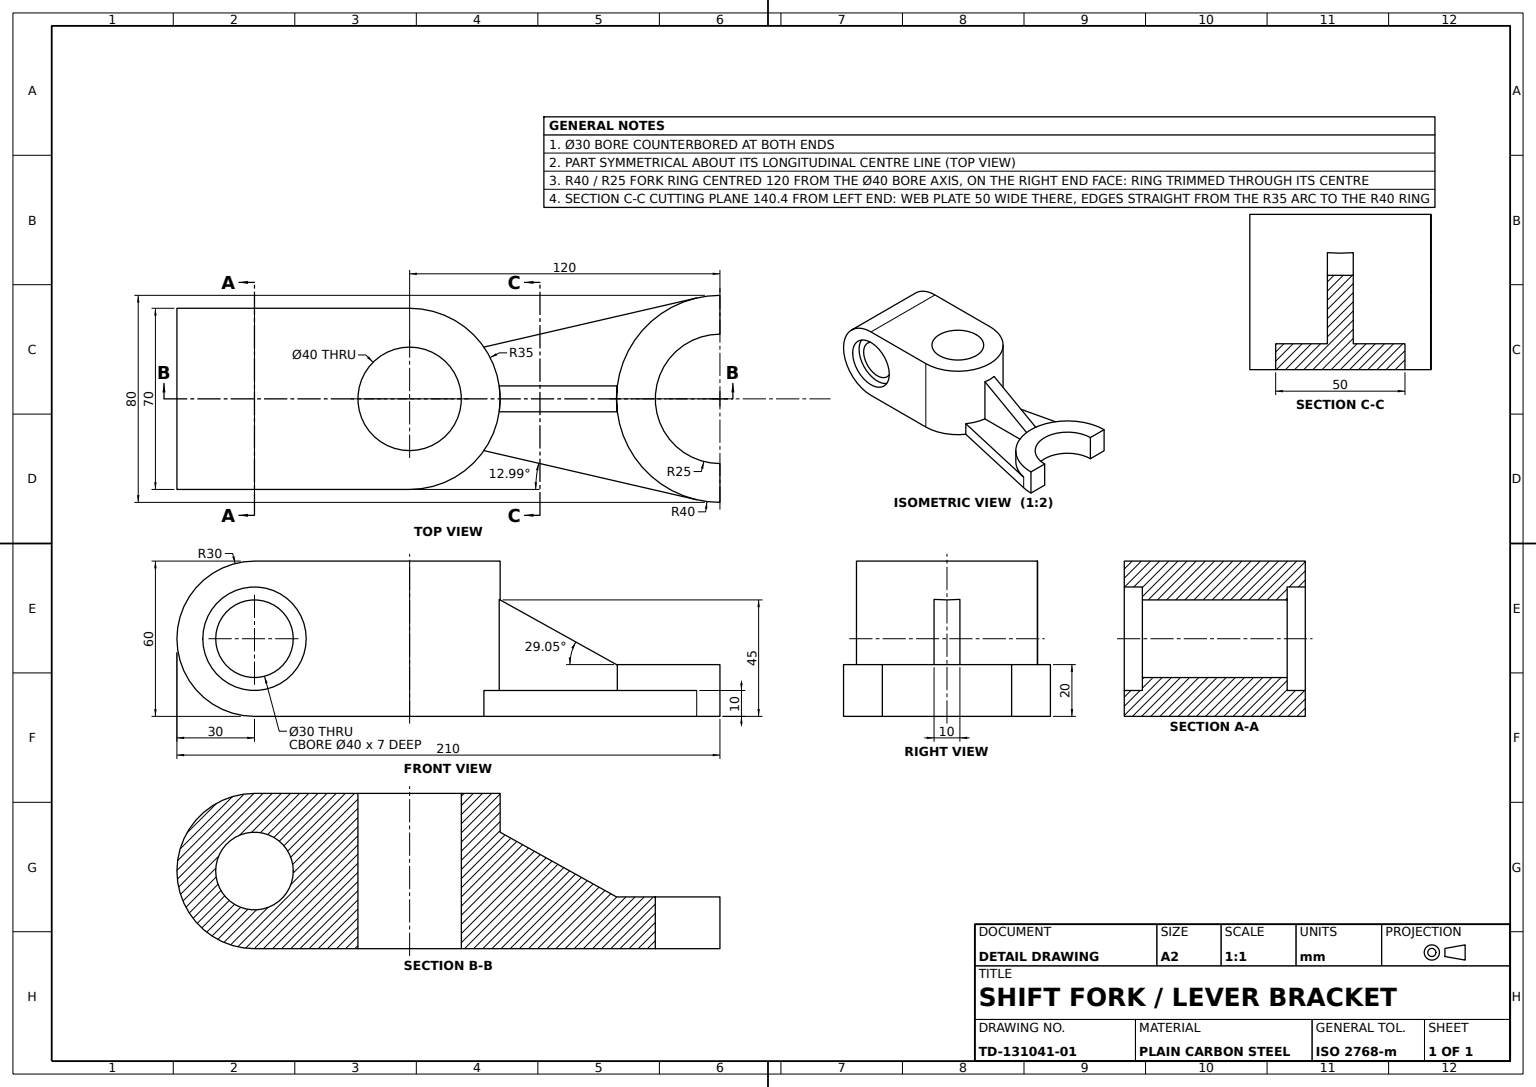
SolidWorks part; units mm, degrees
material "Plain Carbon Steel"
ref_plane "Front Plane" through (0, 0, 0) normal (0, 0, 1) x (1, 0, 0)
ref_plane "Top Plane" through (0, 0, 0) normal (0, 1, 0) x (1, 0, 0)
ref_plane "Right Plane" through (0, 0, 0) normal (1, 0, 0) x (0, 0, -1)
sketch "Base Block Sketch" plane through (0, 0, 0) normal (0, 1, 0) x (1, 0, 0)
  line L0 (0, 35) -> (-90, 35)
  line L1 (-90, 35) -> (-90, -35)
  line L2 (-90, -35) -> (0, -35)
  arc A0 (0, -35) -> (0, 35) centre (0, 0) ccw
  dimension "D1" = 70
  dimension "D2" = 90
extrude "Base Block" add sketch "Base Block Sketch" along normal blind 60
sketch "Block Side Profile Sketch" plane through (0, 0, 35) normal (0, 0, 1) x (1, 0, 0)
  line L0 (-90, 60) -> (-90, 0) construction
  line L1 (-60, 60) -> (-120, 60)
  line L2 (-120, 60) -> (-120, 0)
  line L3 (-120, 0) -> (-60, 0)
  arc A0 (-60, 60) -> (-60, 0) centre (-60, 30) ccw
  point P7 (-90, 30)
  dimension "D1" = 60
  dimension "D2" = 30
  dimension "D3" = 60
extrude "Block Side Profile Cut" cut sketch "Block Side Profile Sketch" against normal through all
sketch "Vertical Bore Sketch" plane through (0, 60, 0) normal (0, 1, 0) x (1, 0, 0)
  circle A0 centre (0, 0) radius 20
  dimension "D1" = 40
extrude "Vertical Bore Ø40" cut sketch "Vertical Bore Sketch" against normal through all
sketch "Horizontal Bore Sketch" plane through (0, 0, 35) normal (0, 0, 1) x (1, 0, 0)
  circle A0 centre (-60, 30) radius 15
  dimension "D1" = 30
extrude "Horizontal Bore Ø30" cut sketch "Horizontal Bore Sketch" against normal through all
sketch "Counterbore Side A Sketch" plane through (0, 0, 35) normal (0, 0, 1) x (1, 0, 0)
  circle A0 centre (-60, 30) radius 20
  dimension "D1" = 40
extrude "Counterbore Side A Ø40x7" cut sketch "Counterbore Side A Sketch" against normal blind 7
sketch "Counterbore Side B Sketch" plane through (0, 0, -35) normal (0, 0, -1) x (-1, 0, 0)
  circle A0 centre (60, 30) radius 20
  dimension "D1" = 40
extrude "Counterbore Side B Ø40x7" cut sketch "Counterbore Side B Sketch" against normal blind 7
sketch "Fork Arm Sketch" plane through (0, 0, 0) normal (0, 1, 0) x (1, 0, 0)
  line L0 (120, 40) -> (120, 25)
  line L1 (120, -25) -> (120, -40)
  arc A0 (120, 40) -> (120, -40) centre (120, 0) ccw
  arc A1 (120, 25) -> (120, -25) centre (120, 0) ccw
  dimension "D1" = 80
  dimension "D2" = 50
  dimension "D3" = 120
extrude "Fork Arm" add sketch "Fork Arm Sketch" along normal blind 20 separate body
sketch "Arm Web Plate Sketch" plane through (0, 0, 0) normal (0, 1, 0) x (1, 0, 0)
  line L0 (111.0113, 38.977) -> (28.7228, 20)
  line L1 (111.0113, -38.977) -> (28.7228, -20)
  arc A0 (28.7228, -20) -> (28.7228, 20) centre (0, 0) ccw
  arc A1 (0, -35) -> (0, 35) centre (0, 0) ccw construction
  arc A2 (111.0113, 38.977) -> (111.0113, -38.977) centre (120, 0) ccw
  dimension "D1" = 80
  dimension "D3" = 40
  dimension "D4" = 20
extrude "Arm Web Plate" add sketch "Arm Web Plate Sketch" along normal blind 10
sketch "Arm Rib Sketch" plane through (0, 0, 0) normal (0, 0, 1) x (1, 0, 0)
  line L0 (35, 10) -> (35, 60) construction
  line L1 (35, 45) -> (80, 20)
  dimension "D1" = 45
rib "Arm Rib" sketch "Arm Rib Sketch" sketch "Arm Rib Sketch" thickness 10 extrusion direction parallel to sketch draft on no parameters "D1"=10
